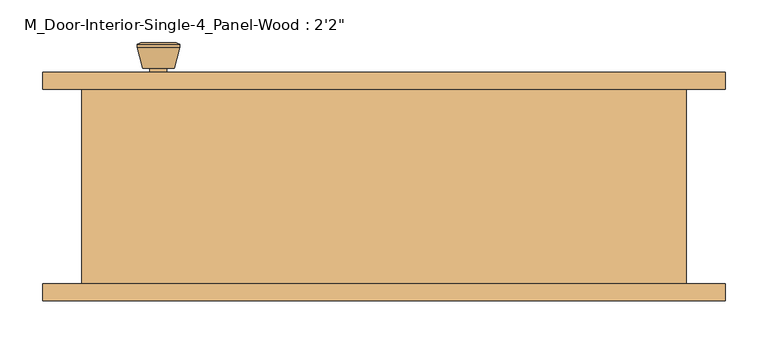
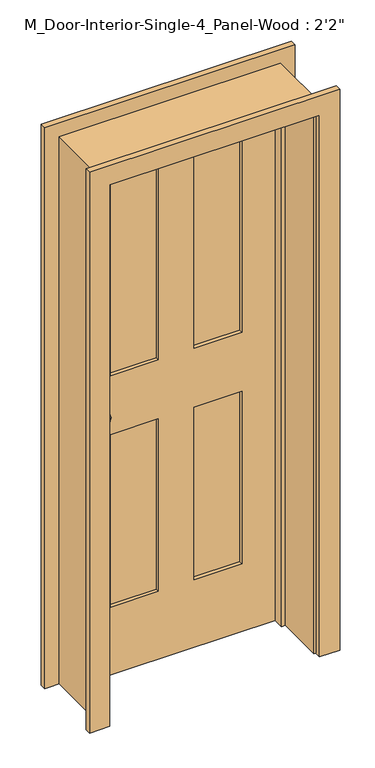
"""IFC4 building model written with IfcOpenShell, lengths in millimetres: door geometry."""

from ifc_helpers import new_model, si_unit, point, frame, frame_2d, origin, place, context, project, spatial, polyline, circle_curve, trimmed, segment, composite_curve, outline, extrude, faceted_brep, source, transform, mapped, element, save
from ifc_brep_helpers import plane_surface, cylinder_surface, revolved_surface, advanced_brep


def door_46909e31(model_context):
    return source(origin(), model_context, "Body", "SolidModel", [
        advanced_brep(
        [(-265.2, 70.125, 914.4), (-255.2, 70.125, 914.4), (-275.2, 70.125, 914.4), (-244.7241324, 21.125, 914.4), (-265.2, 21.125, 914.4), (-285.6758676, 21.125, 914.4), (-240.2, 22.9528681, 914.4), (-290.2, 22.9528681, 914.4), (-240.2, 26.4165463, 914.4), (-290.2, 26.4165463, 914.4), (-246.563764, 51.125, 914.4), (-283.836236, 51.125, 914.4), (-255.2, 51.125, 914.4), (-275.2, 51.125, 914.4)],
        [
            (0, 1),
            (1, 2, circle_curve(frame((-265.2, 70.125, 914.4), z_axis=(0.0, 1.0, 0.0), x_axis=(-1.0, 0.0, 0.0)), 10.0)),
            (2, 0),
            (2, 1, circle_curve(frame((-265.2, 70.125, 914.4), z_axis=(0.0, 1.0, 0.0), x_axis=(-1.0, 0.0, 0.0)), 10.0)),
            (3, 4),
            (4, 5),
            (5, 3, circle_curve(frame((-265.2, 21.125, 914.4), z_axis=(0.0, -1.0, 0.0), x_axis=(-1.0, 0.0, 0.0)), 20.4758676)),
            (3, 5, circle_curve(frame((-265.2, 21.125, 914.4), z_axis=(0.0, -1.0, 0.0), x_axis=(-1.0, 0.0, 0.0)), 20.4758676)),
            (6, 3),
            (5, 7),
            (7, 6, circle_curve(frame((-265.2, 22.9528681, 914.4), z_axis=(0.0, -1.0, 0.0), x_axis=(-1.0, 0.0, 0.0)), 25.0)),
            (6, 7, circle_curve(frame((-265.2, 22.9528681, 914.4), z_axis=(0.0, -1.0, 0.0), x_axis=(-1.0, 0.0, 0.0)), 25.0)),
            (8, 6),
            (7, 9),
            (9, 8, circle_curve(frame((-265.2, 26.4165463, 914.4), z_axis=(0.0, -1.0, 0.0), x_axis=(-1.0, 0.0, 0.0)), 25.0)),
            (8, 9, circle_curve(frame((-265.2, 26.4165463, 914.4), z_axis=(0.0, -1.0, 0.0), x_axis=(-1.0, 0.0, 0.0)), 25.0)),
            (10, 8),
            (9, 11),
            (11, 10, circle_curve(frame((-265.2, 51.125, 914.4), z_axis=(0.0, -1.0, 0.0), x_axis=(-1.0, 0.0, 0.0)), 18.636236)),
            (10, 11, circle_curve(frame((-265.2, 51.125, 914.4), z_axis=(0.0, -1.0, 0.0), x_axis=(-1.0, 0.0, 0.0)), 18.636236)),
            (12, 10),
            (11, 13),
            (13, 12, circle_curve(frame((-265.2, 51.125, 914.4), z_axis=(0.0, -1.0, 0.0), x_axis=(-1.0, 0.0, 0.0)), 10.0)),
            (12, 13, circle_curve(frame((-265.2, 51.125, 914.4), z_axis=(0.0, -1.0, 0.0), x_axis=(-1.0, 0.0, 0.0)), 10.0)),
            (1, 12),
            (13, 2),
        ],
        [
            plane_surface(frame((-265.2, 70.125, 914.4), z_axis=(0.0, 1.0, 0.0), x_axis=(-1.0, 0.0, 0.0))),
            plane_surface(frame((-265.2, 21.125, 914.4), z_axis=(0.0, -1.0, 0.0), x_axis=(-1.0, 0.0, 0.0))),
            revolved_surface(polyline([(-285.6758676, 21.125, 914.4), (-290.2, 22.9528681, 914.4)]), (-265.2, 70.125, 914.4), (0.0, 1.0, 0.0)),
            cylinder_surface(frame((-265.2, 70.125, 914.4), z_axis=(0.0, 1.0, 0.0), x_axis=(-1.0, 0.0, 0.0)), 25.0),
            revolved_surface(polyline([(-290.2, 26.4165463, 914.4), (-283.836236, 51.125, 914.4)]), (-265.2, 70.125, 914.4), (0.0, 1.0, 0.0)),
            plane_surface(frame((-265.2, 51.125, 914.4), z_axis=(0.0, 1.0, 0.0), x_axis=(-1.0, 0.0, 0.0))),
            cylinder_surface(frame((-265.2, 70.125, 914.4), z_axis=(0.0, 1.0, 0.0), x_axis=(-1.0, 0.0, 0.0)), 10.0),
        ],
        [
            (0, [[1, 2, 3]]),
            (0, [[-3, 4, -1]]),
            (1, [[5, 6, 7]]),
            (1, [[-6, -5, 8]]),
            (2, [[9, -7, 10, 11]]),
            (2, [[-10, -8, -9, 12]]),
            (3, [[13, -11, 14, 15]]),
            (3, [[-14, -12, -13, 16]]),
            (4, [[17, -15, 18, 19]]),
            (4, [[-18, -16, -17, 20]]),
            (5, [[21, -19, 22, 23]]),
            (5, [[-22, -20, -21, 24]]),
            (6, [[25, -23, 26, -2]]),
            (6, [[-26, -24, -25, -4]]),
        ],
    ),
        extrude(outline(composite_curve([segment(trimmed(circle_curve(frame_2d((914.4, -265.2)), 30.0), [point((914.4, -295.2))], [point((914.4, -235.2))], False, "CARTESIAN"), True, "CONTINUOUS"), segment(trimmed(circle_curve(frame_2d((914.4, -265.2)), 30.0), [point((914.4, -235.2))], [point((914.4, -295.2))], False, "CARTESIAN"), True, "CONTINUOUS")], self_intersect=False)), frame((0.0, 70.125, 0.0), z_axis=(0.0, 1.0, 0.0), x_axis=(0.0, 0.0, 1.0)), (0.0, 0.0, 1.0), 6.0),
        advanced_brep(
        [(-265.2, 117.125, 914.4), (-275.2, 117.125, 914.4), (-255.2, 117.125, 914.4), (-244.7241324, 166.125, 914.4), (-285.6758676, 166.125, 914.4), (-265.2, 166.125, 914.4), (-240.2, 164.2971319, 914.4), (-290.2, 164.2971319, 914.4), (-240.2, 160.8334537, 914.4), (-290.2, 160.8334537, 914.4), (-246.563764, 136.125, 914.4), (-283.836236, 136.125, 914.4), (-255.2, 136.125, 914.4), (-275.2, 136.125, 914.4)],
        [
            (0, 1),
            (1, 2, circle_curve(frame((-265.2, 117.125, 914.4), z_axis=(0.0, -1.0, 0.0), x_axis=(-1.0, 0.0, 0.0)), 10.0)),
            (2, 0),
            (2, 1, circle_curve(frame((-265.2, 117.125, 914.4), z_axis=(0.0, -1.0, 0.0), x_axis=(-1.0, 0.0, 0.0)), 10.0)),
            (3, 4, circle_curve(frame((-265.2, 166.125, 914.4), z_axis=(0.0, 1.0, 0.0), x_axis=(-1.0, 0.0, 0.0)), 20.4758676)),
            (4, 5),
            (5, 3),
            (4, 3, circle_curve(frame((-265.2, 166.125, 914.4), z_axis=(0.0, 1.0, 0.0), x_axis=(-1.0, 0.0, 0.0)), 20.4758676)),
            (6, 7, circle_curve(frame((-265.2, 164.2971319, 914.4), z_axis=(0.0, 1.0, 0.0), x_axis=(-1.0, 0.0, 0.0)), 25.0)),
            (7, 4),
            (3, 6),
            (7, 6, circle_curve(frame((-265.2, 164.2971319, 914.4), z_axis=(0.0, 1.0, 0.0), x_axis=(-1.0, 0.0, 0.0)), 25.0)),
            (8, 9, circle_curve(frame((-265.2, 160.8334537, 914.4), z_axis=(0.0, 1.0, 0.0), x_axis=(-1.0, 0.0, 0.0)), 25.0)),
            (9, 7),
            (6, 8),
            (9, 8, circle_curve(frame((-265.2, 160.8334537, 914.4), z_axis=(0.0, 1.0, 0.0), x_axis=(-1.0, 0.0, 0.0)), 25.0)),
            (10, 11, circle_curve(frame((-265.2, 136.125, 914.4), z_axis=(0.0, 1.0, 0.0), x_axis=(-1.0, 0.0, 0.0)), 18.636236)),
            (11, 9),
            (8, 10),
            (11, 10, circle_curve(frame((-265.2, 136.125, 914.4), z_axis=(0.0, 1.0, 0.0), x_axis=(-1.0, 0.0, 0.0)), 18.636236)),
            (12, 13, circle_curve(frame((-265.2, 136.125, 914.4), z_axis=(0.0, 1.0, 0.0), x_axis=(-1.0, 0.0, 0.0)), 10.0)),
            (13, 11),
            (10, 12),
            (13, 12, circle_curve(frame((-265.2, 136.125, 914.4), z_axis=(0.0, 1.0, 0.0), x_axis=(-1.0, 0.0, 0.0)), 10.0)),
            (1, 13),
            (12, 2),
        ],
        [
            plane_surface(frame((-265.2, 117.125, 914.4), z_axis=(0.0, -1.0, 0.0), x_axis=(-1.0, 0.0, 0.0))),
            plane_surface(frame((-265.2, 166.125, 914.4), z_axis=(0.0, 1.0, 0.0), x_axis=(-1.0, 0.0, 0.0))),
            revolved_surface(polyline([(-285.6758676, 166.125, 914.4), (-290.2, 164.2971319, 914.4)]), (-265.2, 117.125, 914.4), (0.0, -1.0, 0.0)),
            cylinder_surface(frame((-265.2, 117.125, 914.4), z_axis=(0.0, -1.0, 0.0), x_axis=(-1.0, 0.0, 0.0)), 25.0),
            revolved_surface(polyline([(-290.2, 160.8334537, 914.4), (-283.836236, 136.125, 914.4)]), (-265.2, 117.125, 914.4), (0.0, -1.0, 0.0)),
            plane_surface(frame((-265.2, 136.125, 914.4), z_axis=(0.0, -1.0, 0.0), x_axis=(-1.0, 0.0, 0.0))),
            cylinder_surface(frame((-265.2, 117.125, 914.4), z_axis=(0.0, -1.0, 0.0), x_axis=(-1.0, 0.0, 0.0)), 10.0),
        ],
        [
            (0, [[1, 2, 3]]),
            (0, [[-3, 4, -1]]),
            (1, [[5, 6, 7]]),
            (1, [[8, -7, -6]]),
            (2, [[9, 10, -5, 11]]),
            (2, [[12, -11, -8, -10]]),
            (3, [[13, 14, -9, 15]]),
            (3, [[16, -15, -12, -14]]),
            (4, [[17, 18, -13, 19]]),
            (4, [[20, -19, -16, -18]]),
            (5, [[21, 22, -17, 23]]),
            (5, [[24, -23, -20, -22]]),
            (6, [[-2, 25, -21, 26]]),
            (6, [[-4, -26, -24, -25]]),
        ],
    ),
        extrude(outline(composite_curve([segment(trimmed(circle_curve(frame_2d((914.4, -265.2)), 30.0), [point((914.4, -295.2))], [point((914.4, -235.2))], False, "CARTESIAN"), True, "CONTINUOUS"), segment(trimmed(circle_curve(frame_2d((914.4, -265.2)), 30.0), [point((914.4, -235.2))], [point((914.4, -295.2))], False, "CARTESIAN"), True, "CONTINUOUS")], self_intersect=False)), frame((0.0, 111.125, 0.0), z_axis=(0.0, 1.0, 0.0), x_axis=(0.0, 0.0, 1.0)), (0.0, 0.0, 1.0), 6.0),
        faceted_brep([(355.2, 111.125, 0.0), (355.2, -117.475, 0.0), (330.2, -117.475, 0.0), (330.2, 41.2, 0.0), (317.5, 41.2, 0.0), (317.5, 76.125, 0.0), (330.2, 76.125, 0.0), (330.2, 111.125, 0.0), (355.2, 111.125, 1853.8), (355.2, -117.475, 1853.8), (-355.2, -117.475, 1853.8), (-355.2, -117.475, 0.0), (-330.2, -117.475, 0.0), (-330.2, -117.475, 1828.8), (330.2, -117.475, 1828.8), (330.2, 41.2, 1828.8), (-330.2, 41.2, 1828.8), (-330.2, 41.2, 0.0), (-317.5, 41.2, 0.0), (-317.5, 41.2, 1816.1), (317.5, 41.2, 1816.1), (317.5, 76.125, 1816.1), (-317.5, 76.125, 1816.1), (-317.5, 76.125, 0.0), (-330.2, 76.125, 0.0), (-330.2, 76.125, 1828.8), (330.2, 76.125, 1828.8), (330.2, 111.125, 1828.8), (-330.2, 111.125, 1828.8), (-330.2, 111.125, 0.0), (-355.2, 111.125, 0.0), (-355.2, 111.125, 1853.8)], [[[0, 1, 2, 3, 4, 5, 6, 7]], [[1, 0, 8, 9]], [[2, 1, 9, 10, 11, 12, 13, 14]], [[3, 2, 14, 15]], [[4, 3, 15, 16, 17, 18, 19, 20]], [[5, 4, 20, 21]], [[6, 5, 21, 22, 23, 24, 25, 26]], [[7, 6, 26, 27]], [[0, 7, 27, 28, 29, 30, 31, 8]], [[9, 8, 31, 10]], [[15, 14, 13, 16]], [[21, 20, 19, 22]], [[27, 26, 25, 28]], [[30, 29, 24, 23, 18, 17, 12, 11]], [[10, 31, 30, 11]], [[16, 13, 12, 17]], [[22, 19, 18, 23]], [[28, 25, 24, 29]]]),
        extrude(outline(polyline([(1828.8, -330.2), (0.0, -330.2), (0.0, 330.2), (1828.8, 330.2), (1828.8, -330.2)]), holes=[polyline([(1708.8, 57.5), (1708.8, 210.2), (1014.4, 210.2), (1014.4, 57.5), (1708.8, 57.5)]), polyline([(1014.4, -57.5), (1014.4, -210.2), (1708.8, -210.2), (1708.8, -57.5), (1014.4, -57.5)]), polyline([(814.4, 57.5), (814.4, 210.2), (230.0, 210.2), (230.0, 57.5), (814.4, 57.5)]), polyline([(230.0, -57.5), (230.0, -210.2), (814.4, -210.2), (814.4, -57.5), (230.0, -57.5)])]), frame((0.0, 76.125, 0.0), z_axis=(0.0, 1.0, 0.0), x_axis=(0.0, 0.0, 1.0)), (0.0, 0.0, 1.0), 35.0),
        extrude(outline(polyline([(210.2, 87.7916667), (57.5, 87.7916667), (57.5, 99.4583333), (210.2, 99.4583333), (210.2, 87.7916667)])), frame((0.0, 0.0, 1014.4), z_axis=(0.0, 0.0, 1.0), x_axis=(1.0, 0.0, 0.0)), (0.0, 0.0, 1.0), 694.4),
        extrude(outline(polyline([(-57.5, 87.7916667), (-210.2, 87.7916667), (-210.2, 99.4583333), (-57.5, 99.4583333), (-57.5, 87.7916667)])), frame((0.0, 0.0, 1014.4), z_axis=(0.0, 0.0, 1.0), x_axis=(1.0, 0.0, 0.0)), (0.0, 0.0, 1.0), 694.4),
        extrude(outline(polyline([(210.2, 87.7916667), (57.5, 87.7916667), (57.5, 99.4583333), (210.2, 99.4583333), (210.2, 87.7916667)])), frame((0.0, 0.0, 230.0), z_axis=(0.0, 0.0, 1.0), x_axis=(1.0, 0.0, 0.0)), (0.0, 0.0, 1.0), 584.4),
        extrude(outline(polyline([(-57.5, 87.7916667), (-210.2, 87.7916667), (-210.2, 99.4583333), (-57.5, 99.4583333), (-57.5, 87.7916667)])), frame((0.0, 0.0, 230.0), z_axis=(0.0, 0.0, 1.0), x_axis=(1.0, 0.0, 0.0)), (0.0, 0.0, 1.0), 584.4),
        extrude(outline(polyline([(0.0, 336.55), (0.0, 401.55), (1900.15, 401.55), (1900.15, -401.55), (0.0, -401.55), (0.0, -336.55), (1835.15, -336.55), (1835.15, 336.55), (0.0, 336.55)])), frame((0.0, 111.125, 0.0), z_axis=(0.0, 1.0, 0.0), x_axis=(0.0, 0.0, 1.0)), (0.0, 0.0, 1.0), 20.0),
        extrude(outline(polyline([(0.0, 336.55), (0.0, 401.55), (1900.15, 401.55), (1900.15, -401.55), (0.0, -401.55), (0.0, -336.55), (1835.15, -336.55), (1835.15, 336.55), (0.0, 336.55)])), frame((0.0, -137.475, 0.0), z_axis=(0.0, 1.0, 0.0), x_axis=(0.0, 0.0, 1.0)), (0.0, 0.0, 1.0), 20.0),
    ])


if __name__ == "__main__":
    model = new_model("IFC4")
    model_context = context("Model", 3, world=origin())
    ifc_project = project(units=[si_unit("LENGTHUNIT", "METRE", prefix="MILLI")], contexts=[model_context])
    site = spatial("IfcSite", under=ifc_project)
    building = spatial("IfcBuilding", under=site)
    placement = place(None, origin())
    door_shape = door_46909e31(model_context)
    element("IfcDoor", 1, ObjectType="M_Door-Interior-Single-4_Panel-Wood : 2'2\"", at=placement, inside=building, context=model_context, shape_type="MappedRepresentation", body=[
        mapped(door_shape, transform((0.0, 0.0, 0.0), x_axis=(1.0, 0.0, 0.0), y_axis=(0.0, 1.0, 0.0), z_axis=(0.0, 0.0, 1.0))),
    ])
    save(model, "model.ifc")

# Revit data of these elements
# Type "M_Door-Interior-Single-4_Panel-Wood : 2'2\""
#   Type Mark = "43"
#   Assembly Code = "C1020300"
#   Analytic Construction = "Wooden"
#   Top Rail = 0' - 4.72441"
#   Thickness = 0' - 1.37795"
#   Thermal Resistance (R) = 0.455703 (m²·K)/W
#   Swing Angle [instance default] = 90.00°
#   Stiles = 0' - 4.72441"
#   Rough Width = 2' - 3.9685"
#   Rough Height = 6' - 0.98425"
#   Mullion = 0' - 4.52756"
#   Lock Rail = 0' - 7.87402"
#   Height = 6' - 0"
#   Width = 2' - 2"
#   Heat Transfer Coefficient (U) = 2.19465 W/(m²·K)
#   Bottom Rail = 0' - 9.05512"
#   Trim Material = Cherry
#   Panel Material = Cherry
#   Frame Material = Cherry
#   Door Handle Material = Aluminum
#   Visual Light Transmittance = 0
#   Solar Heat Gain Coefficient = 0
#   Wall Closure = (empty or 0)
#   Function = (empty or 0)
# Element 1 (IfcDoor, "M_Door-Interior-Single-4_Panel-Wood : 2'2\"")
#   Materials on its faces: "Cherry", "Aluminum"
# Materials
#   "Cherry": class "Wood", colour RGB 226 177 128, transparency 0, Description = "Prunus Serotina", Cost = 0
#   "Aluminum": class "Metal", colour RGB 247 247 247, transparency 0, Description = "Aluminum 6061", Cost = 0
